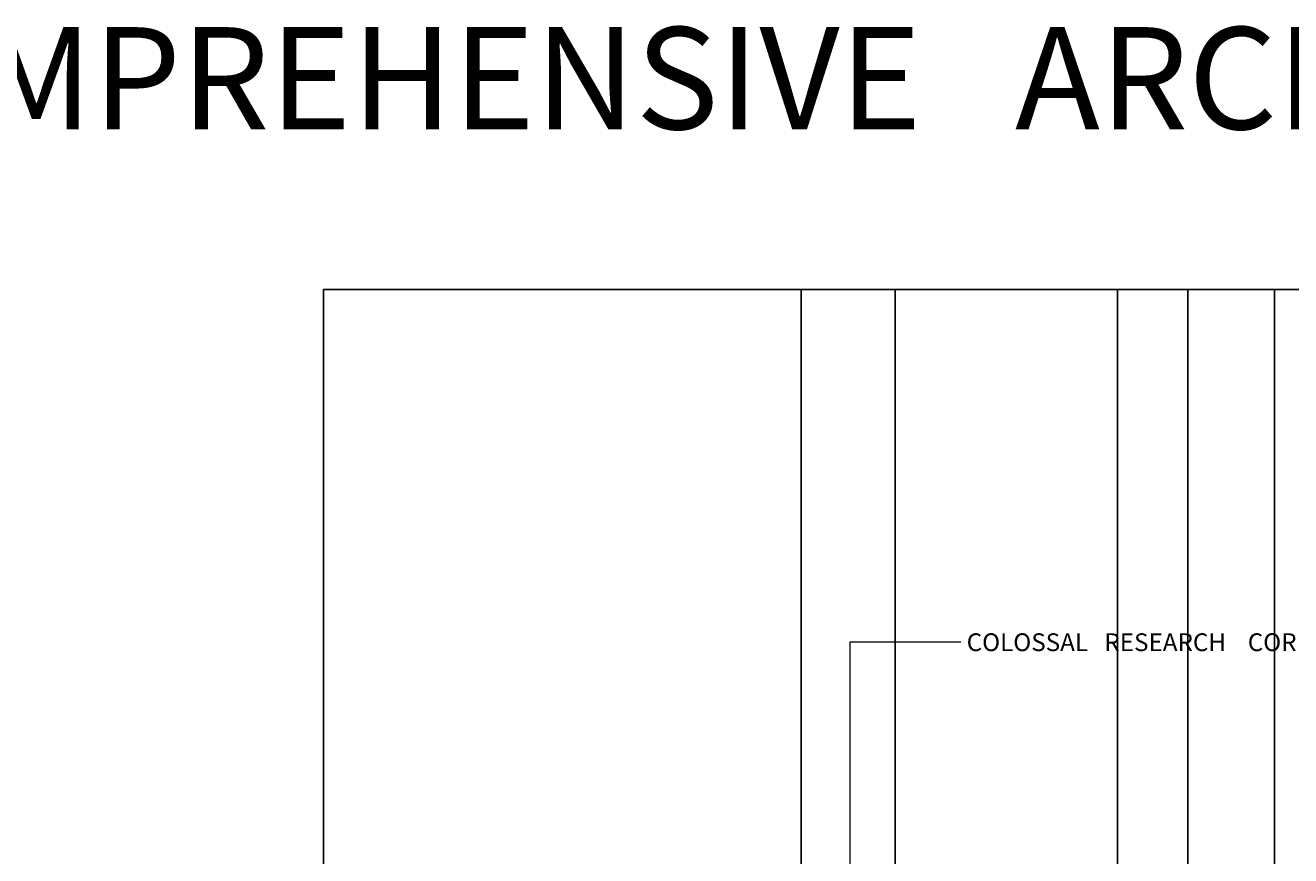
# Model space of a CAD drawing. Units: inches. Extents: x -32109 to 33221, y -19197 to 7608.
# Tile 8 of 25: x -20585 to -11787, y 1836 to 7608. Entities that reach past the tile are written whole.
import ezdxf

# ---------------------------------------------------------------- set-up
doc = ezdxf.new("R2010")
doc.units = ezdxf.units.IN
doc.header["$MEASUREMENT"] = 0
for name, color, linetype, lineweight in [('A-ANNO-DIMS', 2, 'Continuous', 18), ('A-ANNO-NOTE', 2, 'Continuous', 18), ('A-ANNO-TEXT', 7, 'Continuous', 25)]:
    doc.layers.add(name, color=color, linetype=linetype, lineweight=lineweight)
doc.styles.get("Standard").update_dxf_attribs({"font": 'arial.ttf'})
doc.dimstyles.get("Standard").update_dxf_attribs({"dimtxt": 0.18, "dimasz": 0.18, "dimexe": 0.18, "dimexo": 0.0625, "dimgap": 0.09, "dimtad": 0, "dimtih": 1, "dimtoh": 1, "dimdec": 4, "dimzin": 0, "dimdsep": 46, "dimtxsty": 'Standard', "dimcen": 0.09, "dimadec": 0, "dimazin": 0, "dimtfac": 1, "dimtdec": 4, "dimtofl": 0, "dimtmove": 0, "dimatfit": 3, "dimfxl": 1, "dimtolj": 1, "dimtzin": 0, "dimarcsym": 0})

# ---------------------------------------------------------------- blocks, each defined once
blk = doc.blocks.new('*D10')
at = {"layer": 'A-ANNO-DIMS', "color": 0, "lineweight": -2, "transparency": 16777216}
for p, q in [((-18512.646816, -110.179138), (-18512.646816, 5772.015489000001)), ((-18512.466816, 5771.835489), (-202.0927503703958, 5771.835489)), ((18109.136745, 5771.835489), (-201.2373206296045, 5771.835489)), ((18109.316745, -101.537382), (18109.316745, 5772.015489000001))]:
    blk.add_line(p, q, dxfattribs=at)
at = {"layer": 'A-ANNO-DIMS', "color": 0, "transparency": 16777216}
for points in [[(-18512.466816, 5771.865488999999), (-18512.466816, 5771.805489000001), (-18512.646816, 5771.835489)], [(18109.136745, 5771.865488999999), (18109.136745, 5771.805489000001), (18109.316745, 5771.835489)]]:
    blk.add_solid(points, dxfattribs=at)
at = {"layer": 'Defpoints', "color": 0, "transparency": 16777216}
for p in [(18109.316745, 5771.835489), (-18512.646816, -110.241638), (18109.316745, -101.599882)]:
    blk.add_point(p, dxfattribs=at)
at = {"layer": 'A-ANNO-DIMS', "color": 0, "transparency": 16777216, "insert": (-201.6650355000002, 5771.835489), "char_height": 0.18, "attachment_point": 5}
blk.add_mtext('\\A1;36622', dxfattribs=at)
blk = doc.blocks.new('*D32')
at = {"layer": 'A-ANNO-DIMS', "color": 0, "lineweight": -2, "transparency": 16777216}
for p, q in [((-15189.725596, 955.1505220000001), (-15189.725596, 5772.015489000001)), ((-15189.545596, 5771.835489), (-14864.27138008868, 5771.835489)), ((-14538.208774, 5771.835489), (-14863.48298991132, 5771.835489)), ((-14538.028774, 1696.582648), (-14538.028774, 5772.015489))]:
    blk.add_line(p, q, dxfattribs=at)
at = {"layer": 'A-ANNO-DIMS', "color": 0, "transparency": 16777216}
for points in [[(-15189.545596, 5771.865488999999), (-15189.545596, 5771.805489000001), (-15189.725596, 5771.835489)], [(-14538.208774, 5771.865488999999), (-14538.208774, 5771.805489000001), (-14538.028774, 5771.835489)]]:
    blk.add_solid(points, dxfattribs=at)
at = {"layer": 'Defpoints', "color": 0, "transparency": 16777216}
for p in [(-14538.028774, 5771.835489), (-14538.028774, 1696.520148), (-15189.725596, 955.0880219999999)]:
    blk.add_point(p, dxfattribs=at)
at = {"layer": 'A-ANNO-DIMS', "color": 0, "transparency": 16777216, "insert": (-14863.877185, 5771.835489), "char_height": 0.18, "attachment_point": 5}
blk.add_mtext('\\A1;651.7', dxfattribs=at)
blk = doc.blocks.new('*D33')
at = {"layer": 'A-ANNO-DIMS', "color": 0, "lineweight": -2, "transparency": 16777216}
for p, q in [((-14538.028774, 1696.582648), (-14538.028774, 5772.015489)), ((-14537.848774, 5771.835489), (-13764.73509669645, 5771.835489)), ((-12990.709755, 5771.835489), (-13763.82343230355, 5771.835489)), ((-12990.529755, 1696.242222), (-12990.529755, 5772.015489000001))]:
    blk.add_line(p, q, dxfattribs=at)
at = {"layer": 'A-ANNO-DIMS', "color": 0, "transparency": 16777216}
for points in [[(-14537.848774, 5771.865488999999), (-14537.848774, 5771.805489000001), (-14538.028774, 5771.835489)], [(-12990.709755, 5771.865488999999), (-12990.709755, 5771.805489000001), (-12990.529755, 5771.835489)]]:
    blk.add_solid(points, dxfattribs=at)
at = {"layer": 'Defpoints', "color": 0, "transparency": 16777216}
for p in [(-12990.529755, 5771.835489), (-14538.028774, 1696.520148), (-12990.529755, 1696.179722)]:
    blk.add_point(p, dxfattribs=at)
at = {"layer": 'A-ANNO-DIMS', "color": 0, "transparency": 16777216, "insert": (-13764.2792645, 5771.835489), "char_height": 0.18, "attachment_point": 5}
blk.add_mtext('\\A1;1547.5', dxfattribs=at)
blk = doc.blocks.new('*D34')
at = {"layer": 'A-ANNO-DIMS', "color": 0, "lineweight": -2, "transparency": 16777216}
for p, q in [((-12990.529755, 1696.242222), (-12990.529755, 5772.015489000001)), ((-12990.349755, 5771.835489), (-12746.34064218417, 5771.835489)), ((-12501.538719, 5771.835489), (-12745.54783181582, 5771.835489)), ((-12501.358719, 1617.788543), (-12501.358719, 5772.015489000001))]:
    blk.add_line(p, q, dxfattribs=at)
at = {"layer": 'A-ANNO-DIMS', "color": 0, "transparency": 16777216}
for points in [[(-12990.349755, 5771.865488999999), (-12990.349755, 5771.805489000001), (-12990.529755, 5771.835489)], [(-12501.538719, 5771.865488999999), (-12501.538719, 5771.805489000001), (-12501.358719, 5771.835489)]]:
    blk.add_solid(points, dxfattribs=at)
at = {"layer": 'Defpoints', "color": 0, "transparency": 16777216}
for p in [(-12501.358719, 5771.835489), (-12990.529755, 1696.179722), (-12501.358719, 1617.726043)]:
    blk.add_point(p, dxfattribs=at)
at = {"layer": 'A-ANNO-DIMS', "color": 0, "transparency": 16777216, "insert": (-12745.944237, 5771.835489), "char_height": 0.18, "attachment_point": 5}
blk.add_mtext('\\A1;489.2', dxfattribs=at)
blk = doc.blocks.new('*D44')
at = {"layer": 'A-ANNO-DIMS', "color": 0, "lineweight": -2, "transparency": 16777216}
for p, q in [((-12501.358719, 764.249093), (-12501.358719, 5772.015489000001)), ((-12501.178719, 5771.835489), (-9938.977615976126, 5771.835489)), ((-7376.057618000001, 5771.835489), (-9938.258721023878, 5771.835489)), ((-7375.877618000001, 764.249093), (-7375.877618000001, 5772.015489000001))]:
    blk.add_line(p, q, dxfattribs=at)
at = {"layer": 'A-ANNO-DIMS', "color": 0, "transparency": 16777216}
for points in [[(-12501.178719, 5771.865488999999), (-12501.178719, 5771.805489000001), (-12501.358719, 5771.835489)], [(-7376.057618000001, 5771.865488999999), (-7376.057618000001, 5771.805489000001), (-7375.877618000001, 5771.835489)]]:
    blk.add_solid(points, dxfattribs=at)
at = {"layer": 'Defpoints', "color": 0, "transparency": 16777216}
for p in [(-7375.877618000001, 5771.835489), (-12501.358719, 764.186593), (-7375.877618000001, 764.186593)]:
    blk.add_point(p, dxfattribs=at)
at = {"layer": 'A-ANNO-DIMS', "color": 0, "transparency": 16777216, "insert": (-9938.618168500001, 5771.835489), "char_height": 0.18, "attachment_point": 5}
blk.add_mtext('\\A1;5125', dxfattribs=at)
blk = doc.blocks.new('*D45')
at = {"layer": 'A-ANNO-DIMS', "color": 0, "lineweight": -2, "transparency": 16777216}
for p, q in [((-11898.560127, 598.986194), (-11898.560127, 5772.015489000001)), ((-11898.380127, 5771.835489), (-11444.88544065006, 5771.835489)), ((-10990.638094, 5771.835489), (-11444.13278034993, 5771.835489)), ((-10990.458094, 598.060066), (-10990.458094, 5772.015489000001))]:
    blk.add_line(p, q, dxfattribs=at)
at = {"layer": 'A-ANNO-DIMS', "color": 0, "transparency": 16777216}
for points in [[(-11898.380127, 5771.865488999999), (-11898.380127, 5771.805489000001), (-11898.560127, 5771.835489)], [(-10990.638094, 5771.865488999999), (-10990.638094, 5771.805489000001), (-10990.458094, 5771.835489)]]:
    blk.add_solid(points, dxfattribs=at)
at = {"layer": 'Defpoints', "color": 0, "transparency": 16777216}
for p in [(-10990.458094, 5771.835489), (-11898.560127, 598.923694), (-10990.458094, 597.997566)]:
    blk.add_point(p, dxfattribs=at)
at = {"layer": 'A-ANNO-DIMS', "color": 0, "transparency": 16777216, "insert": (-11444.5091105, 5771.835489), "char_height": 0.18, "attachment_point": 5}
blk.add_mtext('\\A1;908.1', dxfattribs=at)

msp = doc.modelspace()

# ---------------------------------------------------------------- linework, layer by layer
at = {"layer": 'A-ANNO-NOTE'}
for p, q in [((-14849.34723911481, 1433.587928212481), (-14849.34723911481, 3321.835488633428)), ((-14849.34723911481, 3321.835488633428), (-14080.10503220442, 3321.835488633428))]:
    msp.add_line(p, q, dxfattribs=at)

# ---------------------------------------------------------------- texts
at = {"layer": 'A-ANNO-TEXT'}
for s, height, p in [('COMPREHENSIVE   ARCHITECTURAL   INTERLOCKING    CUBE   MEGA   CAMPUC   MASTER   PLAN ', 709.7949465747753, (-22238.10681632875, 6885.298304043546)), ('COLOSSAL   RESEARCH    CORE ', 123.5547426012344, (-14039.9432806184, 3257.545255676414))]:
    msp.add_text(s, height=height, dxfattribs=at).set_placement(p)

# ---------------------------------------------------------------- dimensions: what is measured, and where the dimension line sits
at = {"layer": 'A-ANNO-DIMS'}
for base, p1, p2, override, picture, middle in [((18109.316745, 5771.835489), (-18512.646816, -110.241638), (18109.316745, -101.599882), {"dimdec": 0, "dimlfac": 1, "dimrnd": 0, "dimzin": 0, "dimdsep": 46, "dimlunit": 2}, '*D10', (-201.6650355000002, 5771.835489)), ((-14538.028774, 5771.835489), (-15189.725596, 955.0880219999999), (-14538.028774, 1696.520148), {"dimdec": 1, "dimlfac": 1, "dimrnd": 0, "dimzin": 0, "dimdsep": 46, "dimlunit": 2}, '*D32', (-14863.877185, 5771.835489)), ((-12990.529755, 5771.835489), (-14538.028774, 1696.520148), (-12990.529755, 1696.179722), {"dimdec": 1, "dimlfac": 1, "dimrnd": 0, "dimzin": 0, "dimdsep": 46, "dimlunit": 2}, '*D33', (-13764.2792645, 5771.835489)), ((-12501.358719, 5771.835489), (-12990.529755, 1696.179722), (-12501.358719, 1617.726043), {"dimdec": 1, "dimlfac": 1, "dimrnd": 0, "dimzin": 0, "dimdsep": 46, "dimlunit": 2}, '*D34', (-12745.944237, 5771.835489)), ((-7375.877618000001, 5771.835489), (-12501.358719, 764.186593), (-7375.877618000001, 764.186593), {"dimdec": 0, "dimlfac": 1, "dimrnd": 0, "dimzin": 0, "dimdsep": 46, "dimlunit": 2}, '*D44', (-9938.618168500001, 5771.835489)), ((-10990.458094, 5771.835489), (-11898.560127, 598.923694), (-10990.458094, 597.997566), {"dimdec": 1, "dimlfac": 1, "dimrnd": 0, "dimzin": 0, "dimdsep": 46, "dimlunit": 2}, '*D45', (-11444.5091105, 5771.835489))]:
    dim = msp.add_linear_dim(base=base, p1=p1, p2=p2, dimstyle='Standard', override=override, dxfattribs=at)
    dim.commit()
    dim.dimension.update_dxf_attribs({"geometry": picture, "text_midpoint": middle})

doc.saveas('drawing.dxf')
